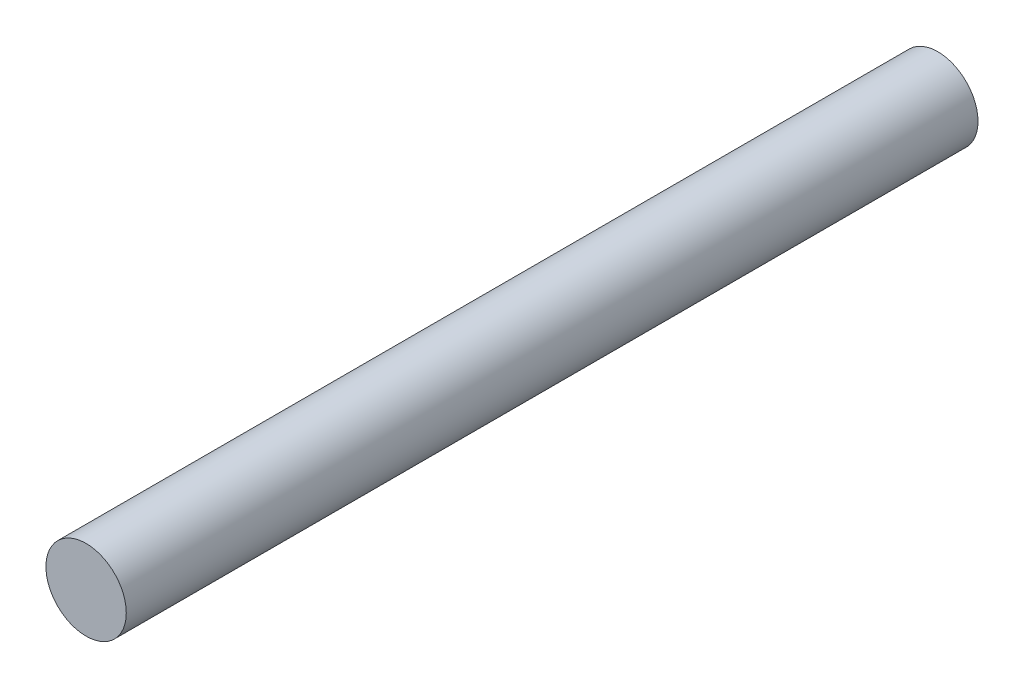
ISO-10303-21;
HEADER;
FILE_DESCRIPTION(('STEP AP214'),'2;1');
FILE_NAME('part.step','',(''),(''),'','','');
FILE_SCHEMA(('AUTOMOTIVE_DESIGN { 1 0 10303 214 1 1 1 1 }'));
ENDSEC;
DATA;
#1=APPLICATION_CONTEXT('core data for automotive mechanical design processes');
#2=APPLICATION_PROTOCOL_DEFINITION('international standard','automotive_design',2000,#1);
#3=PRODUCT_CONTEXT('',#1,'mechanical');
#4=PRODUCT('Part','Part','',(#3));
#5=PRODUCT_RELATED_PRODUCT_CATEGORY('part','',(#4));
#6=PRODUCT_DEFINITION_FORMATION('','',#4);
#7=PRODUCT_DEFINITION_CONTEXT('part definition',#1,'design');
#8=PRODUCT_DEFINITION('design','',#6,#7);
#9=PRODUCT_DEFINITION_SHAPE('','',#8);
#10=(LENGTH_UNIT() NAMED_UNIT(*) SI_UNIT(.MILLI.,.METRE.));
#11=(NAMED_UNIT(*) PLANE_ANGLE_UNIT() SI_UNIT($,.RADIAN.));
#12=(NAMED_UNIT(*) SI_UNIT($,.STERADIAN.) SOLID_ANGLE_UNIT());
#13=UNCERTAINTY_MEASURE_WITH_UNIT(LENGTH_MEASURE(1.E-05),#10,'distance_accuracy_value','');
#14=(GEOMETRIC_REPRESENTATION_CONTEXT(3) GLOBAL_UNCERTAINTY_ASSIGNED_CONTEXT((#13)) GLOBAL_UNIT_ASSIGNED_CONTEXT((#10,
#11,#12)) REPRESENTATION_CONTEXT('',''));
#15=CARTESIAN_POINT('',(0.,0.,0.));
#16=DIRECTION('',(0.,0.,1.));
#17=DIRECTION('',(1.,0.,0.));
#18=AXIS2_PLACEMENT_3D('',#15,#16,#17);
#19=CARTESIAN_POINT('',(0.,0.,26.5));
#20=DIRECTION('',(0.,0.,-1.));
#21=DIRECTION('',(-1.,0.,0.));
#22=AXIS2_PLACEMENT_3D('',#19,#20,#21);
#23=CYLINDRICAL_SURFACE('',#22,2.5);
#24=CARTESIAN_POINT('',(0.,0.,26.5));
#25=DIRECTION('',(0.,0.,1.));
#26=DIRECTION('',(1.,0.,0.));
#27=AXIS2_PLACEMENT_3D('',#24,#25,#26);
#28=CIRCLE('',#27,2.5);
#29=CARTESIAN_POINT('',(2.5,0.,26.5));
#30=VERTEX_POINT('',#29);
#31=EDGE_CURVE('E10',#30,#30,#28,.T.);
#32=ORIENTED_EDGE('',*,*,#31,.F.);
#33=EDGE_LOOP('',(#32));
#34=FACE_BOUND('',#33,.T.);
#35=CARTESIAN_POINT('',(0.,0.,-26.5));
#36=DIRECTION('',(0.,0.,1.));
#37=DIRECTION('',(1.,0.,0.));
#38=AXIS2_PLACEMENT_3D('',#35,#36,#37);
#39=CIRCLE('',#38,2.5);
#40=CARTESIAN_POINT('',(2.5,0.,-26.5));
#41=VERTEX_POINT('',#40);
#42=EDGE_CURVE('E37',#41,#41,#39,.T.);
#43=ORIENTED_EDGE('',*,*,#42,.T.);
#44=EDGE_LOOP('',(#43));
#45=FACE_BOUND('',#44,.T.);
#46=ADVANCED_FACE('F40',(#34,#45),#23,.T.);
#47=CARTESIAN_POINT('',(0.,0.,26.5));
#48=DIRECTION('',(0.,0.,1.));
#49=DIRECTION('',(1.,0.,0.));
#50=AXIS2_PLACEMENT_3D('',#47,#48,#49);
#51=PLANE('',#50);
#52=ORIENTED_EDGE('',*,*,#31,.T.);
#53=EDGE_LOOP('',(#52));
#54=FACE_BOUND('',#53,.T.);
#55=ADVANCED_FACE('F55',(#54),#51,.T.);
#56=CARTESIAN_POINT('',(0.,0.,-26.5));
#57=DIRECTION('',(0.,0.,1.));
#58=DIRECTION('',(1.,0.,0.));
#59=AXIS2_PLACEMENT_3D('',#56,#57,#58);
#60=PLANE('',#59);
#61=ORIENTED_EDGE('',*,*,#42,.F.);
#62=EDGE_LOOP('',(#61));
#63=FACE_BOUND('',#62,.T.);
#64=ADVANCED_FACE('F49',(#63),#60,.F.);
#65=CLOSED_SHELL('',(#46,#55,#64));
#66=MANIFOLD_SOLID_BREP('B2',#65);
#67=ADVANCED_BREP_SHAPE_REPRESENTATION('',(#18,#66),#14);
#68=SHAPE_DEFINITION_REPRESENTATION(#9,#67);
ENDSEC;
END-ISO-10303-21;
